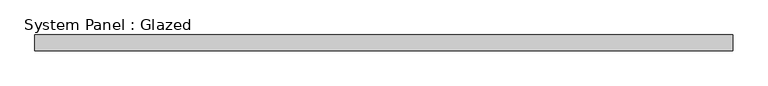
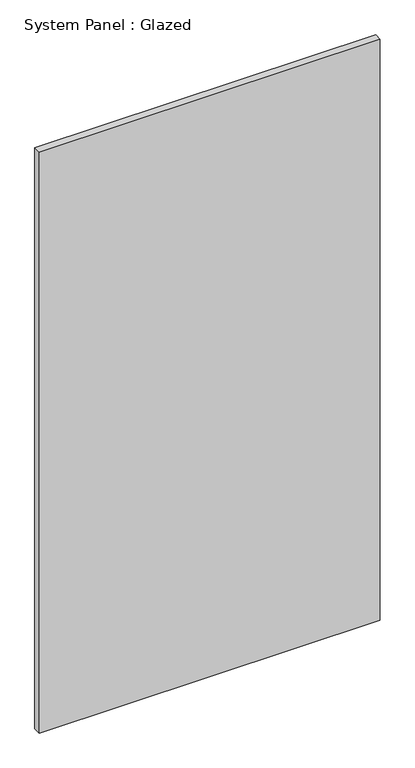
"""IFC4 building model written with IfcOpenShell, lengths in millimetres: plate geometry, System Panel : Glazed."""

from ifc_helpers import new_model, si_unit, origin, origin_with_axes, place, context, project, spatial, polyline, outline, extrude, source, transform, mapped, element, save


def system_panel_glazed_a20b732f(model_context):
    return source(origin(), model_context, "Body", "SweptSolid", [
        extrude(outline(polyline([(565.1499999, 19.05), (-565.1499999, 19.05), (-565.1499999, 44.45), (565.1499999, 44.45), (565.1499999, 19.05)])), origin_with_axes(), (0.0, 0.0, 1.0), 2034.4673659),
    ])


if __name__ == "__main__":
    model = new_model("IFC4")
    model_context = context("Model", 3, world=origin())
    ifc_project = project(units=[si_unit("LENGTHUNIT", "METRE", prefix="MILLI")], contexts=[model_context])
    site = spatial("IfcSite", under=ifc_project)
    building = spatial("IfcBuilding", under=site)
    placement = place(None, origin())
    system_panel_glazed_shape = system_panel_glazed_a20b732f(model_context)
    element("IfcPlate", 1, ObjectType="System Panel : Glazed", at=placement, inside=building, context=model_context, shape_type="MappedRepresentation", body=[
        mapped(system_panel_glazed_shape, transform((0.0, 0.0, 0.0), x_axis=(1.0, 0.0, 0.0), y_axis=(0.0, 1.0, 0.0), z_axis=(0.0, 0.0, 1.0))),
    ])
    save(model, "model.ifc")

# Revit data of these elements
# Type "System Panel : Glazed"
#   Construction Type Id = "GSP4R"
#   Analytic Construction = "1/8 in Pilkington single glazing"
#   Visual Light Transmittance = 0.9
#   Solar Heat Gain Coefficient = 0.86
#   Heat Transfer Coefficient (U) = 1.18115 BTU/(h·ft²·°F)
#   Define Thermal Properties by = 1
# Element 1 (IfcPlate, "System Panel : Glazed")
#   Materials on its faces: "glass panel 223"
# Materials
#   "glass panel 223": class "Generic", colour RGB 120 120 120, transparency 0, Cost = 0
